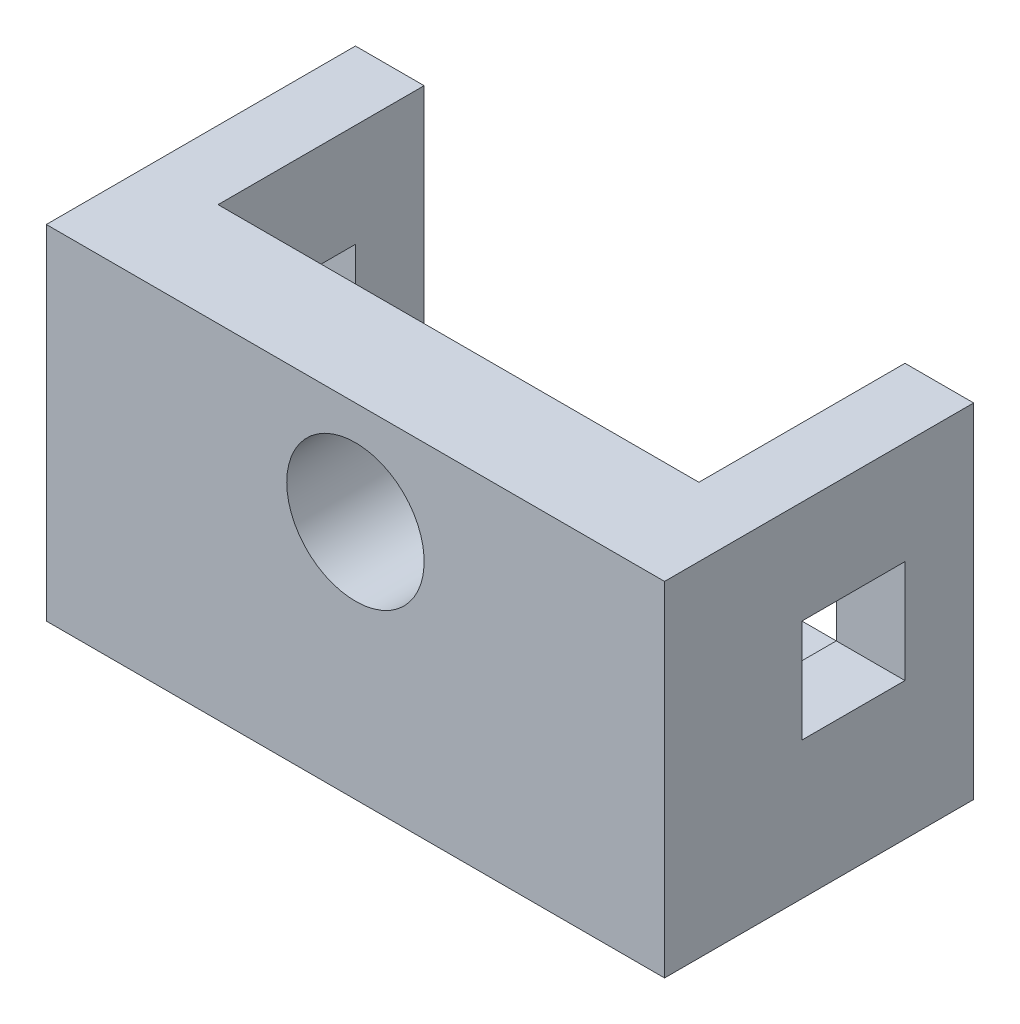
ISO-10303-21;
HEADER;
FILE_DESCRIPTION(('STEP AP214'),'2;1');
FILE_NAME('part.step','',(''),(''),'','','');
FILE_SCHEMA(('AUTOMOTIVE_DESIGN { 1 0 10303 214 1 1 1 1 }'));
ENDSEC;
DATA;
#1=APPLICATION_CONTEXT('core data for automotive mechanical design processes');
#2=APPLICATION_PROTOCOL_DEFINITION('international standard','automotive_design',2000,#1);
#3=PRODUCT_CONTEXT('',#1,'mechanical');
#4=PRODUCT('Part','Part','',(#3));
#5=PRODUCT_RELATED_PRODUCT_CATEGORY('part','',(#4));
#6=PRODUCT_DEFINITION_FORMATION('','',#4);
#7=PRODUCT_DEFINITION_CONTEXT('part definition',#1,'design');
#8=PRODUCT_DEFINITION('design','',#6,#7);
#9=PRODUCT_DEFINITION_SHAPE('','',#8);
#10=(LENGTH_UNIT() NAMED_UNIT(*) SI_UNIT(.MILLI.,.METRE.));
#11=(NAMED_UNIT(*) PLANE_ANGLE_UNIT() SI_UNIT($,.RADIAN.));
#12=(NAMED_UNIT(*) SI_UNIT($,.STERADIAN.) SOLID_ANGLE_UNIT());
#13=UNCERTAINTY_MEASURE_WITH_UNIT(LENGTH_MEASURE(1.E-05),#10,'distance_accuracy_value','');
#14=(GEOMETRIC_REPRESENTATION_CONTEXT(3) GLOBAL_UNCERTAINTY_ASSIGNED_CONTEXT((#13)) GLOBAL_UNIT_ASSIGNED_CONTEXT((#10,
#11,#12)) REPRESENTATION_CONTEXT('',''));
#15=CARTESIAN_POINT('',(0.,0.,0.));
#16=DIRECTION('',(0.,0.,1.));
#17=DIRECTION('',(1.,0.,0.));
#18=AXIS2_PLACEMENT_3D('',#15,#16,#17);
#19=CARTESIAN_POINT('',(-35.,-15.,12.5));
#20=DIRECTION('',(0.,0.,1.));
#21=DIRECTION('',(1.,0.,0.));
#22=AXIS2_PLACEMENT_3D('',#19,#20,#21);
#23=PLANE('',#22);
#24=DIRECTION('',(0.,1.,0.));
#25=VECTOR('',#24,1.);
#26=CARTESIAN_POINT('',(-4.,-15.,12.5));
#27=LINE('',#26,#25);
#28=CARTESIAN_POINT('',(-4.,-15.,12.5));
#29=VERTEX_POINT('',#28);
#30=CARTESIAN_POINT('',(-4.,-9.59591794226542,12.5));
#31=VERTEX_POINT('',#30);
#32=EDGE_CURVE('E219',#29,#31,#27,.T.);
#33=ORIENTED_EDGE('',*,*,#32,.F.);
#34=DIRECTION('',(1.,0.,0.));
#35=VECTOR('',#34,1.);
#36=CARTESIAN_POINT('',(-35.,-15.,12.5));
#37=LINE('',#36,#35);
#38=CARTESIAN_POINT('',(-35.,-15.,12.5));
#39=VERTEX_POINT('',#38);
#40=EDGE_CURVE('E288',#39,#29,#37,.T.);
#41=ORIENTED_EDGE('',*,*,#40,.F.);
#42=DIRECTION('',(0.,1.,0.));
#43=VECTOR('',#42,1.);
#44=CARTESIAN_POINT('',(-35.,-15.,12.5));
#45=LINE('',#44,#43);
#46=CARTESIAN_POINT('',(-35.,10.,12.5));
#47=VERTEX_POINT('',#46);
#48=EDGE_CURVE('E294',#39,#47,#45,.T.);
#49=ORIENTED_EDGE('',*,*,#48,.T.);
#50=DIRECTION('',(-1.,0.,0.));
#51=VECTOR('',#50,1.);
#52=CARTESIAN_POINT('',(-20.,10.,12.5));
#53=LINE('',#52,#51);
#54=CARTESIAN_POINT('',(-20.,10.,12.5));
#55=VERTEX_POINT('',#54);
#56=EDGE_CURVE('E262',#55,#47,#53,.T.);
#57=ORIENTED_EDGE('',*,*,#56,.F.);
#58=CARTESIAN_POINT('',(0.,10.,12.5));
#59=DIRECTION('',(0.,0.,-1.));
#60=DIRECTION('',(-1.,0.,0.));
#61=AXIS2_PLACEMENT_3D('',#58,#59,#60);
#62=CIRCLE('',#61,20.);
#63=EDGE_CURVE('E242',#31,#55,#62,.T.);
#64=ORIENTED_EDGE('',*,*,#63,.F.);
#65=EDGE_LOOP('',(#33,#41,#49,#57,#64));
#66=FACE_BOUND('',#65,.T.);
#67=ADVANCED_FACE('F39',(#66),#23,.F.);
#68=CARTESIAN_POINT('',(0.,-15.,0.));
#69=DIRECTION('',(0.,1.,0.));
#70=DIRECTION('',(0.,0.,1.));
#71=AXIS2_PLACEMENT_3D('',#68,#69,#70);
#72=PLANE('',#71);
#73=ORIENTED_EDGE('',*,*,#40,.T.);
#74=DIRECTION('',(0.,0.,-1.));
#75=VECTOR('',#74,1.);
#76=CARTESIAN_POINT('',(-4.,-15.,0.));
#77=LINE('',#76,#75);
#78=CARTESIAN_POINT('',(-4.,-15.,-22.5));
#79=VERTEX_POINT('',#78);
#80=EDGE_CURVE('E53',#29,#79,#77,.T.);
#81=ORIENTED_EDGE('',*,*,#80,.T.);
#82=DIRECTION('',(-1.,0.,0.));
#83=VECTOR('',#82,1.);
#84=CARTESIAN_POINT('',(-35.,-15.,-22.5));
#85=LINE('',#84,#83);
#86=CARTESIAN_POINT('',(-35.,-15.,-22.5));
#87=VERTEX_POINT('',#86);
#88=EDGE_CURVE('E292',#79,#87,#85,.T.);
#89=ORIENTED_EDGE('',*,*,#88,.T.);
#90=DIRECTION('',(0.,0.,1.));
#91=VECTOR('',#90,1.);
#92=CARTESIAN_POINT('',(-35.,-15.,-22.5));
#93=LINE('',#92,#91);
#94=EDGE_CURVE('E283',#87,#39,#93,.T.);
#95=ORIENTED_EDGE('',*,*,#94,.T.);
#96=EDGE_LOOP('',(#73,#81,#89,#95));
#97=FACE_BOUND('',#96,.T.);
#98=ADVANCED_FACE('F422',(#97),#72,.T.);
#99=CARTESIAN_POINT('',(0.,10.,7.5));
#100=DIRECTION('',(0.,0.,1.));
#101=DIRECTION('',(1.,0.,0.));
#102=AXIS2_PLACEMENT_3D('',#99,#100,#101);
#103=CYLINDRICAL_SURFACE('',#102,20.);
#104=CARTESIAN_POINT('',(20.,10.,12.5));
#105=VERTEX_POINT('',#104);
#106=CARTESIAN_POINT('',(4.,-9.59591794226542,12.5));
#107=VERTEX_POINT('',#106);
#108=EDGE_CURVE('E261',#105,#107,#62,.T.);
#109=ORIENTED_EDGE('',*,*,#108,.T.);
#110=DIRECTION('',(0.,0.,1.));
#111=VECTOR('',#110,1.);
#112=CARTESIAN_POINT('',(4.,-9.59591794226542,7.5));
#113=LINE('',#112,#111);
#114=CARTESIAN_POINT('',(4.,-9.59591794226542,9.92449234640745));
#115=VERTEX_POINT('',#114);
#116=EDGE_CURVE('E11',#107,#115,#113,.F.);
#117=ORIENTED_EDGE('',*,*,#116,.T.);
#118=CARTESIAN_POINT('',(0.,10.,127.5));
#119=DIRECTION('',(0.,-0.986393923832144,0.164398987305357));
#120=DIRECTION('',(0.,0.164398987305357,0.986393923832144));
#121=AXIS2_PLACEMENT_3D('',#118,#119,#120);
#122=ELLIPSE('',#121,121.655250605964,20.);
#123=CARTESIAN_POINT('',(0.,-10.,7.5));
#124=VERTEX_POINT('',#123);
#125=EDGE_CURVE('E50',#115,#124,#122,.F.);
#126=ORIENTED_EDGE('',*,*,#125,.T.);
#127=CARTESIAN_POINT('',(0.,10.,7.5));
#128=DIRECTION('',(0.,0.,-1.));
#129=DIRECTION('',(-1.,0.,0.));
#130=AXIS2_PLACEMENT_3D('',#127,#128,#129);
#131=CIRCLE('',#130,20.);
#132=CARTESIAN_POINT('',(20.,10.,7.5));
#133=VERTEX_POINT('',#132);
#134=EDGE_CURVE('E245',#133,#124,#131,.T.);
#135=ORIENTED_EDGE('',*,*,#134,.F.);
#136=DIRECTION('',(0.,0.,1.));
#137=VECTOR('',#136,1.);
#138=CARTESIAN_POINT('',(20.,10.,7.5));
#139=LINE('',#138,#137);
#140=EDGE_CURVE('E257',#133,#105,#139,.T.);
#141=ORIENTED_EDGE('',*,*,#140,.T.);
#142=EDGE_LOOP('',(#109,#117,#126,#135,#141));
#143=FACE_BOUND('',#142,.T.);
#144=ADVANCED_FACE('F414',(#143),#103,.T.);
#145=CARTESIAN_POINT('',(45.,-5.,-12.5));
#146=DIRECTION('',(0.,0.,1.));
#147=DIRECTION('',(1.,0.,0.));
#148=AXIS2_PLACEMENT_3D('',#145,#146,#147);
#149=PLANE('',#148);
#150=DIRECTION('',(0.,-1.,0.));
#151=VECTOR('',#150,1.);
#152=CARTESIAN_POINT('',(-35.,-5.,-12.5));
#153=LINE('',#152,#151);
#154=CARTESIAN_POINT('',(-35.,10.,-12.5));
#155=VERTEX_POINT('',#154);
#156=CARTESIAN_POINT('',(-35.,-5.,-12.5));
#157=VERTEX_POINT('',#156);
#158=EDGE_CURVE('E320',#155,#157,#153,.T.);
#159=ORIENTED_EDGE('',*,*,#158,.F.);
#160=DIRECTION('',(-1.,0.,0.));
#161=VECTOR('',#160,1.);
#162=CARTESIAN_POINT('',(45.,10.,-12.5));
#163=LINE('',#162,#161);
#164=CARTESIAN_POINT('',(-45.,10.,-12.5));
#165=VERTEX_POINT('',#164);
#166=EDGE_CURVE('E354',#155,#165,#163,.T.);
#167=ORIENTED_EDGE('',*,*,#166,.T.);
#168=DIRECTION('',(0.,1.,0.));
#169=VECTOR('',#168,1.);
#170=CARTESIAN_POINT('',(-45.,-5.,-12.5));
#171=LINE('',#170,#169);
#172=CARTESIAN_POINT('',(-45.,-5.,-12.5));
#173=VERTEX_POINT('',#172);
#174=EDGE_CURVE('E317',#173,#165,#171,.T.);
#175=ORIENTED_EDGE('',*,*,#174,.F.);
#176=DIRECTION('',(-1.,0.,0.));
#177=VECTOR('',#176,1.);
#178=CARTESIAN_POINT('',(45.,-5.,-12.5));
#179=LINE('',#178,#177);
#180=EDGE_CURVE('E329',#157,#173,#179,.T.);
#181=ORIENTED_EDGE('',*,*,#180,.F.);
#182=EDGE_LOOP('',(#159,#167,#175,#181));
#183=FACE_BOUND('',#182,.T.);
#184=ADVANCED_FACE('F411',(#183),#149,.T.);
#185=CARTESIAN_POINT('',(45.,10.,2.5));
#186=DIRECTION('',(0.,-1.,0.));
#187=DIRECTION('',(0.,0.,-1.));
#188=AXIS2_PLACEMENT_3D('',#185,#186,#187);
#189=PLANE('',#188);
#190=DIRECTION('',(0.,0.,-1.));
#191=VECTOR('',#190,1.);
#192=CARTESIAN_POINT('',(-35.,10.,2.49999999999998));
#193=LINE('',#192,#191);
#194=CARTESIAN_POINT('',(-35.,10.,2.5));
#195=VERTEX_POINT('',#194);
#196=EDGE_CURVE('E312',#195,#155,#193,.T.);
#197=ORIENTED_EDGE('',*,*,#196,.F.);
#198=DIRECTION('',(-1.,0.,0.));
#199=VECTOR('',#198,1.);
#200=CARTESIAN_POINT('',(45.,10.,2.5));
#201=LINE('',#200,#199);
#202=CARTESIAN_POINT('',(-45.,10.,2.5));
#203=VERTEX_POINT('',#202);
#204=EDGE_CURVE('E346',#195,#203,#201,.T.);
#205=ORIENTED_EDGE('',*,*,#204,.T.);
#206=DIRECTION('',(0.,0.,1.));
#207=VECTOR('',#206,1.);
#208=CARTESIAN_POINT('',(-45.,10.,2.5));
#209=LINE('',#208,#207);
#210=EDGE_CURVE('E334',#165,#203,#209,.T.);
#211=ORIENTED_EDGE('',*,*,#210,.F.);
#212=ORIENTED_EDGE('',*,*,#166,.F.);
#213=EDGE_LOOP('',(#197,#205,#211,#212));
#214=FACE_BOUND('',#213,.T.);
#215=ADVANCED_FACE('F413',(#214),#189,.T.);
#216=CARTESIAN_POINT('',(45.,-5.,2.5));
#217=DIRECTION('',(0.,0.,-1.));
#218=DIRECTION('',(-1.,0.,0.));
#219=AXIS2_PLACEMENT_3D('',#216,#217,#218);
#220=PLANE('',#219);
#221=DIRECTION('',(0.,1.,0.));
#222=VECTOR('',#221,1.);
#223=CARTESIAN_POINT('',(-35.,-5.,2.5));
#224=LINE('',#223,#222);
#225=CARTESIAN_POINT('',(-35.,-5.,2.5));
#226=VERTEX_POINT('',#225);
#227=EDGE_CURVE('E311',#226,#195,#224,.T.);
#228=ORIENTED_EDGE('',*,*,#227,.F.);
#229=DIRECTION('',(-1.,0.,0.));
#230=VECTOR('',#229,1.);
#231=CARTESIAN_POINT('',(45.,-5.,2.5));
#232=LINE('',#231,#230);
#233=CARTESIAN_POINT('',(-45.,-5.,2.5));
#234=VERTEX_POINT('',#233);
#235=EDGE_CURVE('E342',#226,#234,#232,.T.);
#236=ORIENTED_EDGE('',*,*,#235,.T.);
#237=DIRECTION('',(0.,-1.,0.));
#238=VECTOR('',#237,1.);
#239=CARTESIAN_POINT('',(-45.,-5.,2.5));
#240=LINE('',#239,#238);
#241=EDGE_CURVE('E338',#203,#234,#240,.T.);
#242=ORIENTED_EDGE('',*,*,#241,.F.);
#243=ORIENTED_EDGE('',*,*,#204,.F.);
#244=EDGE_LOOP('',(#228,#236,#242,#243));
#245=FACE_BOUND('',#244,.T.);
#246=ADVANCED_FACE('F402',(#245),#220,.T.);
#247=CARTESIAN_POINT('',(45.,-5.,2.5));
#248=DIRECTION('',(0.,1.,0.));
#249=DIRECTION('',(0.,0.,1.));
#250=AXIS2_PLACEMENT_3D('',#247,#248,#249);
#251=PLANE('',#250);
#252=DIRECTION('',(0.,0.,1.));
#253=VECTOR('',#252,1.);
#254=CARTESIAN_POINT('',(-35.,-5.,2.49999999999998));
#255=LINE('',#254,#253);
#256=EDGE_CURVE('E222',#157,#226,#255,.T.);
#257=ORIENTED_EDGE('',*,*,#256,.F.);
#258=ORIENTED_EDGE('',*,*,#180,.T.);
#259=DIRECTION('',(0.,0.,-1.));
#260=VECTOR('',#259,1.);
#261=CARTESIAN_POINT('',(-45.,-5.,2.5));
#262=LINE('',#261,#260);
#263=EDGE_CURVE('E323',#234,#173,#262,.T.);
#264=ORIENTED_EDGE('',*,*,#263,.F.);
#265=ORIENTED_EDGE('',*,*,#235,.F.);
#266=EDGE_LOOP('',(#257,#258,#264,#265));
#267=FACE_BOUND('',#266,.T.);
#268=ADVANCED_FACE('F404',(#267),#251,.T.);
#269=CARTESIAN_POINT('',(45.,0.,0.));
#270=DIRECTION('',(-1.,0.,0.));
#271=DIRECTION('',(0.,0.,1.));
#272=AXIS2_PLACEMENT_3D('',#269,#270,#271);
#273=PLANE('',#272);
#274=DIRECTION('',(0.,1.,0.));
#275=VECTOR('',#274,1.);
#276=CARTESIAN_POINT('',(45.,-25.,-22.5));
#277=LINE('',#276,#275);
#278=CARTESIAN_POINT('',(45.,-25.,-22.5));
#279=VERTEX_POINT('',#278);
#280=CARTESIAN_POINT('',(45.,25.,-22.5));
#281=VERTEX_POINT('',#280);
#282=EDGE_CURVE('E360',#279,#281,#277,.T.);
#283=ORIENTED_EDGE('',*,*,#282,.T.);
#284=DIRECTION('',(0.,0.,1.));
#285=VECTOR('',#284,1.);
#286=CARTESIAN_POINT('',(45.,25.,22.5));
#287=LINE('',#286,#285);
#288=CARTESIAN_POINT('',(45.,25.,22.5));
#289=VERTEX_POINT('',#288);
#290=EDGE_CURVE('E359',#281,#289,#287,.T.);
#291=ORIENTED_EDGE('',*,*,#290,.T.);
#292=DIRECTION('',(0.,-1.,0.));
#293=VECTOR('',#292,1.);
#294=CARTESIAN_POINT('',(45.,-25.,22.5));
#295=LINE('',#294,#293);
#296=CARTESIAN_POINT('',(45.,-25.,22.5));
#297=VERTEX_POINT('',#296);
#298=EDGE_CURVE('E361',#289,#297,#295,.T.);
#299=ORIENTED_EDGE('',*,*,#298,.T.);
#300=DIRECTION('',(0.,0.,-1.));
#301=VECTOR('',#300,1.);
#302=CARTESIAN_POINT('',(45.,-25.,22.5));
#303=LINE('',#302,#301);
#304=EDGE_CURVE('E364',#297,#279,#303,.T.);
#305=ORIENTED_EDGE('',*,*,#304,.T.);
#306=EDGE_LOOP('',(#283,#291,#299,#305));
#307=FACE_BOUND('',#306,.T.);
#308=DIRECTION('',(0.,1.,0.));
#309=VECTOR('',#308,1.);
#310=CARTESIAN_POINT('',(45.,-5.,-12.5));
#311=LINE('',#310,#309);
#312=CARTESIAN_POINT('',(45.,-5.,-12.5));
#313=VERTEX_POINT('',#312);
#314=CARTESIAN_POINT('',(45.,10.,-12.5));
#315=VERTEX_POINT('',#314);
#316=EDGE_CURVE('E319',#313,#315,#311,.T.);
#317=ORIENTED_EDGE('',*,*,#316,.F.);
#318=DIRECTION('',(0.,0.,-1.));
#319=VECTOR('',#318,1.);
#320=CARTESIAN_POINT('',(45.,-5.,2.5));
#321=LINE('',#320,#319);
#322=CARTESIAN_POINT('',(45.,-5.,2.5));
#323=VERTEX_POINT('',#322);
#324=EDGE_CURVE('E327',#323,#313,#321,.T.);
#325=ORIENTED_EDGE('',*,*,#324,.F.);
#326=DIRECTION('',(0.,-1.,0.));
#327=VECTOR('',#326,1.);
#328=CARTESIAN_POINT('',(45.,-5.,2.5));
#329=LINE('',#328,#327);
#330=CARTESIAN_POINT('',(45.,10.,2.5));
#331=VERTEX_POINT('',#330);
#332=EDGE_CURVE('E324',#331,#323,#329,.T.);
#333=ORIENTED_EDGE('',*,*,#332,.F.);
#334=DIRECTION('',(0.,0.,1.));
#335=VECTOR('',#334,1.);
#336=CARTESIAN_POINT('',(45.,10.,2.5));
#337=LINE('',#336,#335);
#338=EDGE_CURVE('E325',#315,#331,#337,.T.);
#339=ORIENTED_EDGE('',*,*,#338,.F.);
#340=EDGE_LOOP('',(#317,#325,#333,#339));
#341=FACE_BOUND('',#340,.T.);
#342=ADVANCED_FACE('F481',(#307,#341),#273,.F.);
#343=CARTESIAN_POINT('',(-45.,0.,0.));
#344=DIRECTION('',(-1.,0.,0.));
#345=DIRECTION('',(0.,0.,1.));
#346=AXIS2_PLACEMENT_3D('',#343,#344,#345);
#347=PLANE('',#346);
#348=DIRECTION('',(0.,1.,0.));
#349=VECTOR('',#348,1.);
#350=CARTESIAN_POINT('',(-45.,-25.,-22.5));
#351=LINE('',#350,#349);
#352=CARTESIAN_POINT('',(-45.,-25.,-22.5));
#353=VERTEX_POINT('',#352);
#354=CARTESIAN_POINT('',(-45.,25.,-22.5));
#355=VERTEX_POINT('',#354);
#356=EDGE_CURVE('E358',#353,#355,#351,.T.);
#357=ORIENTED_EDGE('',*,*,#356,.F.);
#358=DIRECTION('',(0.,0.,-1.));
#359=VECTOR('',#358,1.);
#360=CARTESIAN_POINT('',(-45.,-25.,22.5));
#361=LINE('',#360,#359);
#362=CARTESIAN_POINT('',(-45.,-25.,22.5));
#363=VERTEX_POINT('',#362);
#364=EDGE_CURVE('E363',#363,#353,#361,.T.);
#365=ORIENTED_EDGE('',*,*,#364,.F.);
#366=DIRECTION('',(0.,-1.,0.));
#367=VECTOR('',#366,1.);
#368=CARTESIAN_POINT('',(-45.,-25.,22.5));
#369=LINE('',#368,#367);
#370=CARTESIAN_POINT('',(-45.,25.,22.5));
#371=VERTEX_POINT('',#370);
#372=EDGE_CURVE('E375',#371,#363,#369,.T.);
#373=ORIENTED_EDGE('',*,*,#372,.F.);
#374=DIRECTION('',(0.,0.,1.));
#375=VECTOR('',#374,1.);
#376=CARTESIAN_POINT('',(-45.,25.,22.5));
#377=LINE('',#376,#375);
#378=EDGE_CURVE('E367',#355,#371,#377,.T.);
#379=ORIENTED_EDGE('',*,*,#378,.F.);
#380=EDGE_LOOP('',(#357,#365,#373,#379));
#381=FACE_BOUND('',#380,.T.);
#382=ORIENTED_EDGE('',*,*,#263,.T.);
#383=ORIENTED_EDGE('',*,*,#174,.T.);
#384=ORIENTED_EDGE('',*,*,#210,.T.);
#385=ORIENTED_EDGE('',*,*,#241,.T.);
#386=EDGE_LOOP('',(#382,#383,#384,#385));
#387=FACE_BOUND('',#386,.T.);
#388=ADVANCED_FACE('F409',(#381,#387),#347,.T.);
#389=CARTESIAN_POINT('',(45.,-25.,-22.5));
#390=DIRECTION('',(0.,0.,1.));
#391=DIRECTION('',(1.,0.,0.));
#392=AXIS2_PLACEMENT_3D('',#389,#390,#391);
#393=PLANE('',#392);
#394=DIRECTION('',(-1.,0.,0.));
#395=VECTOR('',#394,1.);
#396=CARTESIAN_POINT('',(45.,-25.,-22.5));
#397=LINE('',#396,#395);
#398=EDGE_CURVE('E370',#279,#353,#397,.T.);
#399=ORIENTED_EDGE('',*,*,#398,.T.);
#400=ORIENTED_EDGE('',*,*,#356,.T.);
#401=DIRECTION('',(-1.,0.,0.));
#402=VECTOR('',#401,1.);
#403=CARTESIAN_POINT('',(45.,25.,-22.5));
#404=LINE('',#403,#402);
#405=CARTESIAN_POINT('',(-35.,25.,-22.5));
#406=VERTEX_POINT('',#405);
#407=EDGE_CURVE('E382',#406,#355,#404,.T.);
#408=ORIENTED_EDGE('',*,*,#407,.F.);
#409=DIRECTION('',(0.,1.,0.));
#410=VECTOR('',#409,1.);
#411=CARTESIAN_POINT('',(-35.,-15.,-22.5));
#412=LINE('',#411,#410);
#413=EDGE_CURVE('E299',#87,#406,#412,.T.);
#414=ORIENTED_EDGE('',*,*,#413,.F.);
#415=ORIENTED_EDGE('',*,*,#88,.F.);
#416=DIRECTION('',(1.,0.,0.));
#417=VECTOR('',#416,1.);
#418=CARTESIAN_POINT('',(0.,-15.,-22.5));
#419=LINE('',#418,#417);
#420=CARTESIAN_POINT('',(4.,-15.,-22.5));
#421=VERTEX_POINT('',#420);
#422=EDGE_CURVE('E63',#421,#79,#419,.F.);
#423=ORIENTED_EDGE('',*,*,#422,.F.);
#424=CARTESIAN_POINT('',(35.,-15.,-22.5));
#425=VERTEX_POINT('',#424);
#426=EDGE_CURVE('E295',#425,#421,#85,.T.);
#427=ORIENTED_EDGE('',*,*,#426,.F.);
#428=DIRECTION('',(0.,1.,0.));
#429=VECTOR('',#428,1.);
#430=CARTESIAN_POINT('',(35.,-15.,-22.5));
#431=LINE('',#430,#429);
#432=CARTESIAN_POINT('',(35.,25.,-22.5));
#433=VERTEX_POINT('',#432);
#434=EDGE_CURVE('E296',#425,#433,#431,.T.);
#435=ORIENTED_EDGE('',*,*,#434,.T.);
#436=EDGE_CURVE('E383',#281,#433,#404,.T.);
#437=ORIENTED_EDGE('',*,*,#436,.F.);
#438=ORIENTED_EDGE('',*,*,#282,.F.);
#439=EDGE_LOOP('',(#399,#400,#408,#414,#415,#423,#427,#435,#437,#438));
#440=FACE_BOUND('',#439,.T.);
#441=ADVANCED_FACE('F41',(#440),#393,.F.);
#442=CARTESIAN_POINT('',(45.,25.,22.5));
#443=DIRECTION('',(0.,-1.,0.));
#444=DIRECTION('',(0.,0.,-1.));
#445=AXIS2_PLACEMENT_3D('',#442,#443,#444);
#446=PLANE('',#445);
#447=DIRECTION('',(0.,0.,-1.));
#448=VECTOR('',#447,1.);
#449=CARTESIAN_POINT('',(35.,25.,-22.5));
#450=LINE('',#449,#448);
#451=CARTESIAN_POINT('',(35.,25.,7.5));
#452=VERTEX_POINT('',#451);
#453=EDGE_CURVE('E281',#452,#433,#450,.T.);
#454=ORIENTED_EDGE('',*,*,#453,.F.);
#455=DIRECTION('',(1.,0.,0.));
#456=VECTOR('',#455,1.);
#457=CARTESIAN_POINT('',(35.,25.,7.5));
#458=LINE('',#457,#456);
#459=CARTESIAN_POINT('',(-35.,25.,7.5));
#460=VERTEX_POINT('',#459);
#461=EDGE_CURVE('E252',#460,#452,#458,.T.);
#462=ORIENTED_EDGE('',*,*,#461,.F.);
#463=DIRECTION('',(0.,0.,1.));
#464=VECTOR('',#463,1.);
#465=CARTESIAN_POINT('',(-35.,25.,-22.5));
#466=LINE('',#465,#464);
#467=EDGE_CURVE('E278',#406,#460,#466,.T.);
#468=ORIENTED_EDGE('',*,*,#467,.F.);
#469=ORIENTED_EDGE('',*,*,#407,.T.);
#470=ORIENTED_EDGE('',*,*,#378,.T.);
#471=DIRECTION('',(-1.,0.,0.));
#472=VECTOR('',#471,1.);
#473=CARTESIAN_POINT('',(45.,25.,22.5));
#474=LINE('',#473,#472);
#475=EDGE_CURVE('E379',#289,#371,#474,.T.);
#476=ORIENTED_EDGE('',*,*,#475,.F.);
#477=ORIENTED_EDGE('',*,*,#290,.F.);
#478=ORIENTED_EDGE('',*,*,#436,.T.);
#479=EDGE_LOOP('',(#454,#462,#468,#469,#470,#476,#477,#478));
#480=FACE_BOUND('',#479,.T.);
#481=ADVANCED_FACE('F474',(#480),#446,.F.);
#482=CARTESIAN_POINT('',(45.,-25.,22.5));
#483=DIRECTION('',(0.,0.,-1.));
#484=DIRECTION('',(-1.,0.,0.));
#485=AXIS2_PLACEMENT_3D('',#482,#483,#484);
#486=PLANE('',#485);
#487=ORIENTED_EDGE('',*,*,#372,.T.);
#488=DIRECTION('',(-1.,0.,0.));
#489=VECTOR('',#488,1.);
#490=CARTESIAN_POINT('',(45.,-25.,22.5));
#491=LINE('',#490,#489);
#492=EDGE_CURVE('E378',#297,#363,#491,.T.);
#493=ORIENTED_EDGE('',*,*,#492,.F.);
#494=ORIENTED_EDGE('',*,*,#298,.F.);
#495=ORIENTED_EDGE('',*,*,#475,.T.);
#496=EDGE_LOOP('',(#487,#493,#494,#495));
#497=FACE_BOUND('',#496,.T.);
#498=CARTESIAN_POINT('',(0.,10.,22.5));
#499=DIRECTION('',(0.,0.,-1.));
#500=DIRECTION('',(-1.,0.,0.));
#501=AXIS2_PLACEMENT_3D('',#498,#499,#500);
#502=CIRCLE('',#501,10.);
#503=CARTESIAN_POINT('',(-10.,10.,22.5));
#504=VERTEX_POINT('',#503);
#505=EDGE_CURVE('E240',#504,#504,#502,.F.);
#506=ORIENTED_EDGE('',*,*,#505,.F.);
#507=EDGE_LOOP('',(#506));
#508=FACE_BOUND('',#507,.T.);
#509=ADVANCED_FACE('F494',(#497,#508),#486,.F.);
#510=CARTESIAN_POINT('',(45.,-25.,22.5));
#511=DIRECTION('',(0.,1.,0.));
#512=DIRECTION('',(0.,0.,1.));
#513=AXIS2_PLACEMENT_3D('',#510,#511,#512);
#514=PLANE('',#513);
#515=ORIENTED_EDGE('',*,*,#492,.T.);
#516=ORIENTED_EDGE('',*,*,#364,.T.);
#517=ORIENTED_EDGE('',*,*,#398,.F.);
#518=ORIENTED_EDGE('',*,*,#304,.F.);
#519=EDGE_LOOP('',(#515,#516,#517,#518));
#520=FACE_BOUND('',#519,.T.);
#521=ADVANCED_FACE('F429',(#520),#514,.F.);
#522=DIRECTION('',(0.,1.,0.));
#523=VECTOR('',#522,1.);
#524=CARTESIAN_POINT('',(35.,-5.,-12.5));
#525=LINE('',#524,#523);
#526=CARTESIAN_POINT('',(35.,-5.,-12.5));
#527=VERTEX_POINT('',#526);
#528=CARTESIAN_POINT('',(35.,10.,-12.5));
#529=VERTEX_POINT('',#528);
#530=EDGE_CURVE('E313',#527,#529,#525,.T.);
#531=ORIENTED_EDGE('',*,*,#530,.F.);
#532=EDGE_CURVE('E343',#313,#527,#179,.T.);
#533=ORIENTED_EDGE('',*,*,#532,.F.);
#534=ORIENTED_EDGE('',*,*,#316,.T.);
#535=EDGE_CURVE('E352',#315,#529,#163,.T.);
#536=ORIENTED_EDGE('',*,*,#535,.T.);
#537=EDGE_LOOP('',(#531,#533,#534,#536));
#538=FACE_BOUND('',#537,.T.);
#539=ADVANCED_FACE('F417',(#538),#149,.T.);
#540=DIRECTION('',(0.,0.,1.));
#541=VECTOR('',#540,1.);
#542=CARTESIAN_POINT('',(35.,10.,2.5));
#543=LINE('',#542,#541);
#544=CARTESIAN_POINT('',(35.,10.,2.5));
#545=VERTEX_POINT('',#544);
#546=EDGE_CURVE('E310',#529,#545,#543,.T.);
#547=ORIENTED_EDGE('',*,*,#546,.F.);
#548=ORIENTED_EDGE('',*,*,#535,.F.);
#549=ORIENTED_EDGE('',*,*,#338,.T.);
#550=EDGE_CURVE('E349',#331,#545,#201,.T.);
#551=ORIENTED_EDGE('',*,*,#550,.T.);
#552=EDGE_LOOP('',(#547,#548,#549,#551));
#553=FACE_BOUND('',#552,.T.);
#554=ADVANCED_FACE('F421',(#553),#189,.T.);
#555=DIRECTION('',(0.,-1.,0.));
#556=VECTOR('',#555,1.);
#557=CARTESIAN_POINT('',(35.,-5.,2.5));
#558=LINE('',#557,#556);
#559=CARTESIAN_POINT('',(35.,-5.,2.5));
#560=VERTEX_POINT('',#559);
#561=EDGE_CURVE('E300',#545,#560,#558,.T.);
#562=ORIENTED_EDGE('',*,*,#561,.F.);
#563=ORIENTED_EDGE('',*,*,#550,.F.);
#564=ORIENTED_EDGE('',*,*,#332,.T.);
#565=EDGE_CURVE('E344',#323,#560,#232,.T.);
#566=ORIENTED_EDGE('',*,*,#565,.T.);
#567=EDGE_LOOP('',(#562,#563,#564,#566));
#568=FACE_BOUND('',#567,.T.);
#569=ADVANCED_FACE('F622',(#568),#220,.T.);
#570=DIRECTION('',(0.,0.,-1.));
#571=VECTOR('',#570,1.);
#572=CARTESIAN_POINT('',(35.,-5.,2.5));
#573=LINE('',#572,#571);
#574=EDGE_CURVE('E390',#560,#527,#573,.T.);
#575=ORIENTED_EDGE('',*,*,#574,.F.);
#576=ORIENTED_EDGE('',*,*,#565,.F.);
#577=ORIENTED_EDGE('',*,*,#324,.T.);
#578=ORIENTED_EDGE('',*,*,#532,.T.);
#579=EDGE_LOOP('',(#575,#576,#577,#578));
#580=FACE_BOUND('',#579,.T.);
#581=ADVANCED_FACE('F605',(#580),#251,.T.);
#582=CARTESIAN_POINT('',(-35.,-15.,-22.5));
#583=DIRECTION('',(-1.,0.,0.));
#584=DIRECTION('',(0.,0.,1.));
#585=AXIS2_PLACEMENT_3D('',#582,#583,#584);
#586=PLANE('',#585);
#587=ORIENTED_EDGE('',*,*,#158,.T.);
#588=ORIENTED_EDGE('',*,*,#256,.T.);
#589=ORIENTED_EDGE('',*,*,#227,.T.);
#590=ORIENTED_EDGE('',*,*,#196,.T.);
#591=EDGE_LOOP('',(#587,#588,#589,#590));
#592=FACE_BOUND('',#591,.T.);
#593=ORIENTED_EDGE('',*,*,#467,.T.);
#594=DIRECTION('',(0.,1.,0.));
#595=VECTOR('',#594,1.);
#596=CARTESIAN_POINT('',(-35.,25.,7.5));
#597=LINE('',#596,#595);
#598=CARTESIAN_POINT('',(-35.,10.,7.5));
#599=VERTEX_POINT('',#598);
#600=EDGE_CURVE('E247',#599,#460,#597,.T.);
#601=ORIENTED_EDGE('',*,*,#600,.F.);
#602=DIRECTION('',(0.,0.,1.));
#603=VECTOR('',#602,1.);
#604=CARTESIAN_POINT('',(-35.,10.,7.5));
#605=LINE('',#604,#603);
#606=EDGE_CURVE('E274',#599,#47,#605,.T.);
#607=ORIENTED_EDGE('',*,*,#606,.T.);
#608=ORIENTED_EDGE('',*,*,#48,.F.);
#609=ORIENTED_EDGE('',*,*,#94,.F.);
#610=ORIENTED_EDGE('',*,*,#413,.T.);
#611=EDGE_LOOP('',(#593,#601,#607,#608,#609,#610));
#612=FACE_BOUND('',#611,.T.);
#613=ADVANCED_FACE('F394',(#592,#612),#586,.F.);
#614=CARTESIAN_POINT('',(35.,-15.,-22.5));
#615=DIRECTION('',(1.,0.,0.));
#616=DIRECTION('',(0.,0.,-1.));
#617=AXIS2_PLACEMENT_3D('',#614,#615,#616);
#618=PLANE('',#617);
#619=ORIENTED_EDGE('',*,*,#530,.T.);
#620=ORIENTED_EDGE('',*,*,#546,.T.);
#621=ORIENTED_EDGE('',*,*,#561,.T.);
#622=ORIENTED_EDGE('',*,*,#574,.T.);
#623=EDGE_LOOP('',(#619,#620,#621,#622));
#624=FACE_BOUND('',#623,.T.);
#625=DIRECTION('',(0.,0.,1.));
#626=VECTOR('',#625,1.);
#627=CARTESIAN_POINT('',(35.,10.,7.5));
#628=LINE('',#627,#626);
#629=CARTESIAN_POINT('',(35.,10.,7.5));
#630=VERTEX_POINT('',#629);
#631=CARTESIAN_POINT('',(35.,10.,12.5));
#632=VERTEX_POINT('',#631);
#633=EDGE_CURVE('E275',#630,#632,#628,.T.);
#634=ORIENTED_EDGE('',*,*,#633,.F.);
#635=DIRECTION('',(0.,-1.,0.));
#636=VECTOR('',#635,1.);
#637=CARTESIAN_POINT('',(35.,10.,7.5));
#638=LINE('',#637,#636);
#639=EDGE_CURVE('E254',#452,#630,#638,.T.);
#640=ORIENTED_EDGE('',*,*,#639,.F.);
#641=ORIENTED_EDGE('',*,*,#453,.T.);
#642=ORIENTED_EDGE('',*,*,#434,.F.);
#643=DIRECTION('',(0.,0.,-1.));
#644=VECTOR('',#643,1.);
#645=CARTESIAN_POINT('',(35.,-15.,-22.5));
#646=LINE('',#645,#644);
#647=CARTESIAN_POINT('',(35.,-15.,12.5));
#648=VERTEX_POINT('',#647);
#649=EDGE_CURVE('E286',#648,#425,#646,.T.);
#650=ORIENTED_EDGE('',*,*,#649,.F.);
#651=DIRECTION('',(0.,1.,0.));
#652=VECTOR('',#651,1.);
#653=CARTESIAN_POINT('',(35.,-15.,12.5));
#654=LINE('',#653,#652);
#655=EDGE_CURVE('E301',#648,#632,#654,.T.);
#656=ORIENTED_EDGE('',*,*,#655,.T.);
#657=EDGE_LOOP('',(#634,#640,#641,#642,#650,#656));
#658=FACE_BOUND('',#657,.T.);
#659=ADVANCED_FACE('F443',(#624,#658),#618,.F.);
#660=CARTESIAN_POINT('',(4.,-15.,12.5));
#661=VERTEX_POINT('',#660);
#662=EDGE_CURVE('E285',#661,#648,#37,.T.);
#663=ORIENTED_EDGE('',*,*,#662,.F.);
#664=DIRECTION('',(0.,1.,0.));
#665=VECTOR('',#664,1.);
#666=CARTESIAN_POINT('',(4.,-15.,12.5));
#667=LINE('',#666,#665);
#668=EDGE_CURVE('E233',#661,#107,#667,.T.);
#669=ORIENTED_EDGE('',*,*,#668,.T.);
#670=ORIENTED_EDGE('',*,*,#108,.F.);
#671=DIRECTION('',(-1.,0.,0.));
#672=VECTOR('',#671,1.);
#673=CARTESIAN_POINT('',(20.,10.,12.5));
#674=LINE('',#673,#672);
#675=EDGE_CURVE('E270',#632,#105,#674,.T.);
#676=ORIENTED_EDGE('',*,*,#675,.F.);
#677=ORIENTED_EDGE('',*,*,#655,.F.);
#678=EDGE_LOOP('',(#663,#669,#670,#676,#677));
#679=FACE_BOUND('',#678,.T.);
#680=ADVANCED_FACE('F434',(#679),#23,.F.);
#681=DIRECTION('',(0.,0.,-1.));
#682=VECTOR('',#681,1.);
#683=CARTESIAN_POINT('',(4.,-15.,0.));
#684=LINE('',#683,#682);
#685=EDGE_CURVE('E231',#661,#421,#684,.T.);
#686=ORIENTED_EDGE('',*,*,#685,.F.);
#687=ORIENTED_EDGE('',*,*,#662,.T.);
#688=ORIENTED_EDGE('',*,*,#649,.T.);
#689=ORIENTED_EDGE('',*,*,#426,.T.);
#690=EDGE_LOOP('',(#686,#687,#688,#689));
#691=FACE_BOUND('',#690,.T.);
#692=ADVANCED_FACE('F442',(#691),#72,.T.);
#693=CARTESIAN_POINT('',(0.,10.,7.5));
#694=DIRECTION('',(0.,0.,-1.));
#695=DIRECTION('',(-1.,0.,0.));
#696=AXIS2_PLACEMENT_3D('',#693,#694,#695);
#697=PLANE('',#696);
#698=ORIENTED_EDGE('',*,*,#134,.T.);
#699=CARTESIAN_POINT('',(-20.,10.,7.5));
#700=VERTEX_POINT('',#699);
#701=EDGE_CURVE('E209',#124,#700,#131,.T.);
#702=ORIENTED_EDGE('',*,*,#701,.T.);
#703=DIRECTION('',(-1.,0.,0.));
#704=VECTOR('',#703,1.);
#705=CARTESIAN_POINT('',(-20.,10.,7.5));
#706=LINE('',#705,#704);
#707=EDGE_CURVE('E248',#700,#599,#706,.T.);
#708=ORIENTED_EDGE('',*,*,#707,.T.);
#709=ORIENTED_EDGE('',*,*,#600,.T.);
#710=ORIENTED_EDGE('',*,*,#461,.T.);
#711=ORIENTED_EDGE('',*,*,#639,.T.);
#712=DIRECTION('',(-1.,0.,0.));
#713=VECTOR('',#712,1.);
#714=CARTESIAN_POINT('',(20.,10.,7.5));
#715=LINE('',#714,#713);
#716=EDGE_CURVE('E256',#630,#133,#715,.T.);
#717=ORIENTED_EDGE('',*,*,#716,.T.);
#718=EDGE_LOOP('',(#698,#702,#708,#709,#710,#711,#717));
#719=FACE_BOUND('',#718,.T.);
#720=CARTESIAN_POINT('',(0.,10.,7.5));
#721=DIRECTION('',(0.,0.,-1.));
#722=DIRECTION('',(-1.,0.,0.));
#723=AXIS2_PLACEMENT_3D('',#720,#721,#722);
#724=CIRCLE('',#723,10.);
#725=CARTESIAN_POINT('',(-10.,10.,7.5));
#726=VERTEX_POINT('',#725);
#727=EDGE_CURVE('E238',#726,#726,#724,.T.);
#728=ORIENTED_EDGE('',*,*,#727,.F.);
#729=EDGE_LOOP('',(#728));
#730=FACE_BOUND('',#729,.T.);
#731=ADVANCED_FACE('F453',(#719,#730),#697,.T.);
#732=ORIENTED_EDGE('',*,*,#701,.F.);
#733=CARTESIAN_POINT('',(-4.,-9.59591794226542,9.92449234640744));
#734=VERTEX_POINT('',#733);
#735=EDGE_CURVE('E204',#124,#734,#122,.F.);
#736=ORIENTED_EDGE('',*,*,#735,.T.);
#737=DIRECTION('',(0.,0.,1.));
#738=VECTOR('',#737,1.);
#739=CARTESIAN_POINT('',(-4.,-9.59591794226542,7.5));
#740=LINE('',#739,#738);
#741=EDGE_CURVE('E210',#31,#734,#740,.F.);
#742=ORIENTED_EDGE('',*,*,#741,.F.);
#743=ORIENTED_EDGE('',*,*,#63,.T.);
#744=DIRECTION('',(0.,0.,1.));
#745=VECTOR('',#744,1.);
#746=CARTESIAN_POINT('',(-20.,10.,7.5));
#747=LINE('',#746,#745);
#748=EDGE_CURVE('E280',#700,#55,#747,.T.);
#749=ORIENTED_EDGE('',*,*,#748,.F.);
#750=EDGE_LOOP('',(#732,#736,#742,#743,#749));
#751=FACE_BOUND('',#750,.T.);
#752=ADVANCED_FACE('F206',(#751),#103,.T.);
#753=CARTESIAN_POINT('',(-20.,10.,7.5));
#754=DIRECTION('',(0.,1.,0.));
#755=DIRECTION('',(0.,0.,1.));
#756=AXIS2_PLACEMENT_3D('',#753,#754,#755);
#757=PLANE('',#756);
#758=ORIENTED_EDGE('',*,*,#56,.T.);
#759=ORIENTED_EDGE('',*,*,#606,.F.);
#760=ORIENTED_EDGE('',*,*,#707,.F.);
#761=ORIENTED_EDGE('',*,*,#748,.T.);
#762=EDGE_LOOP('',(#758,#759,#760,#761));
#763=FACE_BOUND('',#762,.T.);
#764=ADVANCED_FACE('F507',(#763),#757,.F.);
#765=CARTESIAN_POINT('',(20.,10.,7.5));
#766=DIRECTION('',(0.,1.,0.));
#767=DIRECTION('',(0.,0.,1.));
#768=AXIS2_PLACEMENT_3D('',#765,#766,#767);
#769=PLANE('',#768);
#770=ORIENTED_EDGE('',*,*,#675,.T.);
#771=ORIENTED_EDGE('',*,*,#140,.F.);
#772=ORIENTED_EDGE('',*,*,#716,.F.);
#773=ORIENTED_EDGE('',*,*,#633,.T.);
#774=EDGE_LOOP('',(#770,#771,#772,#773));
#775=FACE_BOUND('',#774,.T.);
#776=ADVANCED_FACE('F468',(#775),#769,.F.);
#777=CARTESIAN_POINT('',(0.,10.,7.5));
#778=DIRECTION('',(0.,0.,1.));
#779=DIRECTION('',(1.,0.,0.));
#780=AXIS2_PLACEMENT_3D('',#777,#778,#779);
#781=CYLINDRICAL_SURFACE('',#780,10.);
#782=ORIENTED_EDGE('',*,*,#727,.T.);
#783=EDGE_LOOP('',(#782));
#784=FACE_BOUND('',#783,.T.);
#785=ORIENTED_EDGE('',*,*,#505,.T.);
#786=EDGE_LOOP('',(#785));
#787=FACE_BOUND('',#786,.T.);
#788=ADVANCED_FACE('F503',(#784,#787),#781,.F.);
#789=CARTESIAN_POINT('',(0.,-10.,7.5));
#790=DIRECTION('',(0.,-0.986393923832144,0.164398987305357));
#791=DIRECTION('',(0.,-0.164398987305357,-0.986393923832144));
#792=AXIS2_PLACEMENT_3D('',#789,#790,#791);
#793=PLANE('',#792);
#794=DIRECTION('',(0.,-0.164398987305357,-0.986393923832144));
#795=VECTOR('',#794,1.);
#796=CARTESIAN_POINT('',(4.,-10.,7.5));
#797=LINE('',#796,#795);
#798=EDGE_CURVE('E223',#115,#421,#797,.T.);
#799=ORIENTED_EDGE('',*,*,#798,.T.);
#800=ORIENTED_EDGE('',*,*,#422,.T.);
#801=DIRECTION('',(0.,-0.164398987305357,-0.986393923832144));
#802=VECTOR('',#801,1.);
#803=CARTESIAN_POINT('',(-4.,-10.,7.5));
#804=LINE('',#803,#802);
#805=EDGE_CURVE('E218',#734,#79,#804,.T.);
#806=ORIENTED_EDGE('',*,*,#805,.F.);
#807=ORIENTED_EDGE('',*,*,#735,.F.);
#808=ORIENTED_EDGE('',*,*,#125,.F.);
#809=EDGE_LOOP('',(#799,#800,#806,#807,#808));
#810=FACE_BOUND('',#809,.T.);
#811=ADVANCED_FACE('F221',(#810),#793,.F.);
#812=CARTESIAN_POINT('',(4.,0.,0.));
#813=DIRECTION('',(1.,0.,0.));
#814=DIRECTION('',(0.,0.,-1.));
#815=AXIS2_PLACEMENT_3D('',#812,#813,#814);
#816=PLANE('',#815);
#817=ORIENTED_EDGE('',*,*,#668,.F.);
#818=ORIENTED_EDGE('',*,*,#685,.T.);
#819=ORIENTED_EDGE('',*,*,#798,.F.);
#820=ORIENTED_EDGE('',*,*,#116,.F.);
#821=EDGE_LOOP('',(#817,#818,#819,#820));
#822=FACE_BOUND('',#821,.T.);
#823=ADVANCED_FACE('F463',(#822),#816,.T.);
#824=CARTESIAN_POINT('',(-4.,0.,0.));
#825=DIRECTION('',(1.,0.,0.));
#826=DIRECTION('',(0.,0.,-1.));
#827=AXIS2_PLACEMENT_3D('',#824,#825,#826);
#828=PLANE('',#827);
#829=ORIENTED_EDGE('',*,*,#80,.F.);
#830=ORIENTED_EDGE('',*,*,#32,.T.);
#831=ORIENTED_EDGE('',*,*,#741,.T.);
#832=ORIENTED_EDGE('',*,*,#805,.T.);
#833=EDGE_LOOP('',(#829,#830,#831,#832));
#834=FACE_BOUND('',#833,.T.);
#835=ADVANCED_FACE('F217',(#834),#828,.F.);
#836=CLOSED_SHELL('',(#67,#98,#144,#184,#215,#246,#268,#342,#388,#441,#481,#509,#521,#539,#554,
#569,#581,#613,#659,#680,#692,#731,#752,#764,#776,#788,#811,#823,#835));
#837=MANIFOLD_SOLID_BREP('B2',#836);
#838=ADVANCED_BREP_SHAPE_REPRESENTATION('',(#18,#837),#14);
#839=SHAPE_DEFINITION_REPRESENTATION(#9,#838);
ENDSEC;
END-ISO-10303-21;
